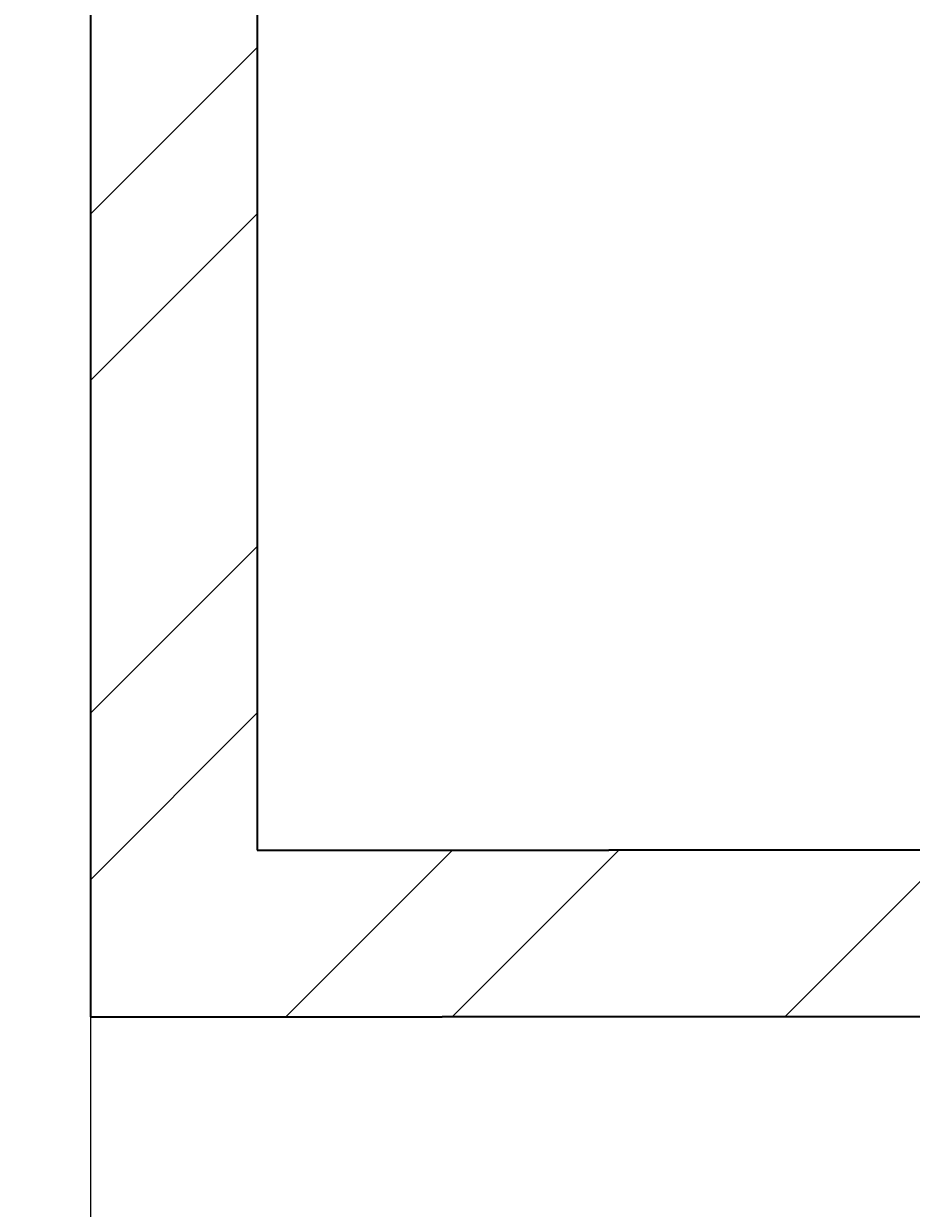
# Model space of a CAD drawing. Units: inches. Extents: x 1885 to 2748, y 783 to 2421.
# Tile 4 of 117: x 1969 to 1993, y 1082 to 1114. Entities that reach past the tile are written whole.
import ezdxf

# ---------------------------------------------------------------- set-up
doc = ezdxf.new("R2010")
doc.units = ezdxf.units.IN
for name, color, linetype, lineweight in [('A-ANNO-DIMS', 2, 'Continuous', 18), ('A-FLOR-BALC', 7, 'Continuous', 25), ('A-WALL', 7, 'Continuous', 35)]:
    doc.layers.add(name, color=color, linetype=linetype, lineweight=lineweight)
doc.layers.add('A-WALL-PATT', color=85, linetype='Continuous', lineweight=13, true_color=0x58ba48)
doc.styles.get("Standard").update_dxf_attribs({"font": 'arial.ttf'})
doc.dimstyles.get("Standard").update_dxf_attribs({"dimtxt": 0.18, "dimasz": 0.18, "dimexe": 0.18, "dimexo": 0.0625, "dimgap": 0.09, "dimtad": 0, "dimtih": 1, "dimtoh": 1, "dimdec": 4, "dimzin": 0, "dimdsep": 46, "dimtxsty": 'Standard', "dimcen": 0.09, "dimadec": 0, "dimazin": 0, "dimtfac": 1, "dimtdec": 4, "dimtofl": 0, "dimtmove": 0, "dimatfit": 3, "dimfxl": 1, "dimtolj": 1, "dimtzin": 0, "dimarcsym": 0})

# ---------------------------------------------------------------- blocks, each defined once
blk = doc.blocks.new('*D45')
at = {"layer": 'A-ANNO-DIMS', "color": 0, "lineweight": -2, "transparency": 16777216}
for p, q in [((1980.711, 1524.006), (1902.844, 1524.006)), ((1903.024, 1523.826), (1903.024, 1290.937)), ((1903.024, 1057.686), (1903.024, 1290.574)), ((1971.211, 1057.506), (1902.844, 1057.506))]:
    blk.add_line(p, q, dxfattribs=at)
at = {"layer": 'A-ANNO-DIMS', "color": 0, "transparency": 16777216}
for points in [[(1902.994, 1523.826), (1903.054, 1523.826), (1903.024, 1524.006)], [(1902.994, 1057.686), (1903.054, 1057.686), (1903.024, 1057.506)]]:
    blk.add_solid(points, dxfattribs=at)
at = {"layer": 'Defpoints', "color": 0, "transparency": 16777216}
for p in [(1903.024, 1524.006), (1980.774, 1524.006), (1971.274, 1057.506)]:
    blk.add_point(p, dxfattribs=at)
at = {"layer": 'A-ANNO-DIMS', "color": 0, "transparency": 16777216, "insert": (1903.024, 1290.756), "char_height": 0.18, "attachment_point": 5}
blk.add_mtext('\\A1;466.5', dxfattribs=at)

msp = doc.modelspace()

# ---------------------------------------------------------------- hatches: boundary and pattern name
at = {"layer": 'A-WALL-PATT'}
h = msp.add_hatch(dxfattribs=at)
h.set_pattern_fill('ANSI32', color=256)
h.paths.add_polyline_path([(2007.772, 2318.006), (1980.774, 2318.006), (1980.774, 2281.215), (1985.274, 2281.215), (1985.274, 2313.506), (2007.772, 2313.506), (2007.772, 2315.756)])
h.paths.add_polyline_path([(2094.324, 2318.006), (2067.772, 2318.006), (2067.772, 2313.506), (2094.324, 2313.506), (2094.324, 2315.756)])
h.paths.add_polyline_path([(2131.367, 2315.756), (2131.367, 2318.006), (2131.189, 2318.006), (2112.609, 2318.006), (2112.609, 2313.506), (2117.274, 2313.506), (2117.274, 2255.201), (2121.774, 2255.201), (2121.774, 2313.506), (2131.367, 2313.506)])
h.paths.add_polyline_path([(2190.512, 2318.006), (2155.367, 2318.006), (2155.367, 2313.506), (2169.774, 2313.506), (2169.774, 2229.506), (2121.774, 2229.506), (2121.774, 2233.451), (2119.524, 2233.451), (2117.274, 2233.451), (2117.274, 2201.101), (2121.774, 2201.101), (2121.774, 2225.006), (2169.774, 2225.006), (2169.774, 2165.006), (2306.274, 2165.006), (2306.274, 2066.006), (2310.774, 2066.006), (2344.274, 2066.006), (2486.274, 2066.006), (2486.274, 1886.006), (2483.02, 1886.006), (2483.02, 1881.506), (2486.274, 1881.506), (2486.274, 1880.678), (2490.774, 1880.678), (2490.774, 2070.506), (2344.274, 2070.506), (2310.774, 2070.506), (2310.774, 2165.006), (2310.774, 2173.636), (2308.524, 2173.636), (2306.274, 2173.636), (2306.274, 2169.506), (2174.274, 2169.506), (2174.274, 2313.506), (2190.512, 2313.506), (2190.512, 2315.756)])
h.paths.add_polyline_path([(1985.274, 2221.215), (1980.774, 2221.215), (1980.774, 2165.006), (1992.774, 2165.006), (1992.774, 2141.927), (1997.274, 2141.927), (1997.274, 2165.006), (2117.274, 2165.006), (2117.274, 2163.126), (2121.774, 2163.126), (2121.774, 2172.734), (2119.524, 2172.734), (2117.274, 2172.734), (2117.274, 2169.506), (1985.274, 2169.506)])
h.paths.add_polyline_path([(1997.274, 2105.927), (1992.774, 2105.927), (1992.774, 2070.506), (2016.774, 2070.506), (2016.774, 2059.123), (2019.024, 2059.123), (2021.274, 2059.123), (2021.274, 2070.506), (2117.274, 2070.506), (2117.274, 2022.506), (2114.423, 2022.506), (2114.423, 2018.006), (2123.627, 2018.006), (2123.627, 2020.256), (2123.627, 2022.506), (2121.774, 2022.506), (2121.774, 2142.587), (2119.524, 2142.587), (2117.274, 2142.587), (2117.274, 2075.006), (1997.274, 2075.006)])
h.paths.add_polyline_path([(2092.029, 2020.256), (2092.029, 2022.506), (2021.274, 2022.506), (2021.274, 2035.123), (2016.774, 2035.123), (2016.774, 2018.006), (2016.774, 1978.784), (2021.274, 1978.784), (2021.274, 2018.006), (2092.029, 2018.006)])
h.paths.add_polyline_path([(2260.938, 2022.506), (2153.105, 2022.506), (2153.105, 2020.256), (2153.105, 2018.006), (2155.274, 2018.006), (2155.274, 1886.006), (2107.629, 1886.006), (2107.629, 1881.506), (2182.911, 1881.506), (2182.911, 1883.756), (2182.911, 1886.006), (2159.774, 1886.006), (2159.774, 2018.006), (2260.938, 2018.006), (2260.938, 2020.256)])
h.paths.add_polyline_path([(2047.629, 1883.756), (2047.629, 1886.006), (2021.274, 1886.006), (2021.274, 1918.784), (2019.024, 1918.784), (2016.774, 1918.784), (2016.774, 1881.506), (2047.629, 1881.506)])
h.paths.add_polyline_path([(2306.361, 1883.756), (2306.361, 1886.006), (2296.274, 1886.006), (2296.274, 1982.006), (2316.535, 1982.006), (2316.535, 1984.256), (2316.535, 1986.506), (2296.274, 1986.506), (2296.274, 2022.506), (2289.276, 2022.506), (2289.276, 2018.006), (2291.774, 2018.006), (2291.774, 1886.006), (2242.911, 1886.006), (2242.911, 1881.506), (2306.361, 1881.506)], flags=17)
h.paths.add_polyline_path([(1985.274, 1843.006), (2021.6, 1843.006), (2021.534, 1845.441), (2021.477, 1847.506), (1980.774, 1847.506), (1980.774, 1809.446), (1985.274, 1809.446)])
h.paths.add_polyline_path([(2131.482, 1845.256), (2131.482, 1847.506), (2081.534, 1847.506), (2081.534, 1843.006), (2117.274, 1843.006), (2117.274, 1784.147), (2119.524, 1784.147), (2121.774, 1784.147), (2121.774, 1843.006), (2131.482, 1843.006)])
h.paths.add_polyline_path([(2203.886, 1847.506), (2155.482, 1847.506), (2155.482, 1843.006), (2169.774, 1843.006), (2169.774, 1759.006), (2121.774, 1759.006), (2121.774, 1761.457), (2117.274, 1761.457), (2117.274, 1730.429), (2121.774, 1730.429), (2121.774, 1754.506), (2177.421, 1754.506), (2177.421, 1756.756), (2177.421, 1759.006), (2174.274, 1759.006), (2174.274, 1843.006), (2203.886, 1843.006)])
h.paths.add_polyline_path([(2335.554, 1845.256), (2335.554, 1847.506), (2239.886, 1847.506), (2239.886, 1843.006), (2306.274, 1843.006), (2306.274, 1759.006), (2199.486, 1759.006), (2199.486, 1754.506), (2310.774, 1754.506), (2310.774, 1843.006), (2335.554, 1843.006)])
h.paths.add_polyline_path([(2348.774, 2022.506), (2344.274, 2022.506), (2344.274, 1986.506), (2341.681, 1986.506), (2341.681, 1982.006), (2344.274, 1982.006), (2344.274, 1886.006), (2330.361, 1886.006), (2330.361, 1881.506), (2361.627, 1881.506), (2361.627, 1883.756), (2361.627, 1886.006), (2348.774, 1886.006)], flags=17)
h.paths.add_polyline_path([(2283.251, 2315.756), (2283.251, 2318.006), (2238.512, 2318.006), (2238.512, 2313.506), (2283.251, 2313.506)], flags=17)
h.paths.add_polyline_path([(2363.274, 2348.006), (2388.677, 2348.006), (2388.677, 2350.256), (2388.677, 2352.506), (2358.774, 2352.506), (2358.774, 2348.006), (2358.774, 2318.006), (2344.481, 2318.006), (2344.481, 2313.506), (2358.774, 2313.506), (2358.774, 2229.506), (2310.774, 2229.506), (2310.774, 2231.952), (2306.274, 2231.952), (2306.274, 2205.611), (2310.774, 2205.611), (2310.774, 2225.006), (2358.774, 2225.006), (2358.774, 2211.506), (2452.329, 2211.506), (2452.329, 2213.756), (2452.329, 2216.006), (2363.274, 2216.006), (2363.274, 2318.006)])
h.paths.add_polyline_path([(2310.774, 2313.506), (2320.481, 2313.506), (2320.481, 2315.756), (2320.481, 2318.006), (2302.728, 2318.006), (2302.728, 2313.506), (2306.274, 2313.506), (2306.274, 2251.076), (2310.774, 2251.076)], flags=17)
h.paths.add_polyline_path([(2490.774, 2352.506), (2486.274, 2352.506), (2448.677, 2352.506), (2448.677, 2348.006), (2486.274, 2348.006), (2486.274, 2318.006), (2486.274, 2216.006), (2481.78, 2216.006), (2481.78, 2211.506), (2486.274, 2211.506), (2486.274, 2165.006), (2493.289, 2165.006), (2493.289, 2167.256), (2493.289, 2169.506), (2490.774, 2169.506), (2490.774, 2313.506), (2494.429, 2313.506), (2494.429, 2318.006), (2490.774, 2318.006)])
h.paths.add_polyline_path([(2534.653, 2318.006), (2515.691, 2318.006), (2515.691, 2313.506), (2534.653, 2313.506), (2534.653, 2315.756)])
h.paths.add_polyline_path([(2618.274, 2318.006), (2594.653, 2318.006), (2594.653, 2313.506), (2613.774, 2313.506), (2613.774, 2281.706), (2618.274, 2281.706)])
h.paths.add_polyline_path([(2618.274, 2221.706), (2613.774, 2221.706), (2613.774, 2169.506), (2554.019, 2169.506), (2554.019, 2165.006), (2613.774, 2165.006), (2613.774, 2152.878), (2618.274, 2152.878)])
h.paths.add_polyline_path([(2618.274, 2128.878), (2616.024, 2128.878), (2613.774, 2128.878), (2613.774, 2117.006), (2529.774, 2117.006), (2529.774, 2165.006), (2532.848, 2165.006), (2532.848, 2169.506), (2522.867, 2169.506), (2522.867, 2165.006), (2525.274, 2165.006), (2525.274, 2117.006), (2525.274, 2112.506), (2525.274, 2108.576), (2529.774, 2108.576), (2529.774, 2112.506), (2613.774, 2112.506), (2613.774, 2080.19), (2618.274, 2080.19)])
h.paths.add_polyline_path([(2618.274, 2044.19), (2616.024, 2044.19), (2613.774, 2044.19), (2613.774, 2015.506), (2529.774, 2015.506), (2529.774, 2088.582), (2527.524, 2088.582), (2525.274, 2088.582), (2525.274, 2011.006), (2613.774, 2011.006), (2613.774, 1956.755), (2618.274, 1956.755)])
h.paths.add_polyline_path([(2618.274, 1881.506), (2618.274, 1896.755), (2613.774, 1896.755), (2613.774, 1881.506), (2613.774, 1847.506), (2592.715, 1847.506), (2592.715, 1843.006), (2613.774, 1843.006), (2613.774, 1765.006), (2613.774, 1760.506), (2609.621, 1760.506), (2609.621, 1756.006), (2613.774, 1756.006), (2613.774, 1660.006), (2608.544, 1660.006), (2608.544, 1655.506), (2613.774, 1655.506), (2613.774, 1508.158), (2618.274, 1508.158)])
h.paths.add_polyline_path([(2565.774, 1843.006), (2568.997, 1843.006), (2568.997, 1847.506), (2490.774, 1847.506), (2490.774, 1849.7), (2488.524, 1849.7), (2486.274, 1849.7), (2486.274, 1847.506), (2477.274, 1847.506), (2477.274, 1838.506), (2477.274, 1821.493), (2486.274, 1821.493), (2486.274, 1838.506), (2561.274, 1838.506), (2561.274, 1765.006), (2486.274, 1765.006), (2486.274, 1786.157), (2477.274, 1786.157), (2477.274, 1765.006), (2477.274, 1756.006), (2486.274, 1756.006), (2565.774, 1756.006), (2585.621, 1756.006), (2585.621, 1758.256), (2585.621, 1760.506), (2565.774, 1760.506), (2565.774, 1765.006)])
h.paths.add_polyline_path([(2486.274, 1651.006), (2561.274, 1651.006), (2561.274, 1567.006), (2486.274, 1567.006), (2486.274, 1591.321), (2477.274, 1591.321), (2477.274, 1567.006), (2477.274, 1558.006), (2477.274, 1555.439), (2481.774, 1555.439), (2481.774, 1558.006), (2568.653, 1558.006), (2568.653, 1560.256), (2568.653, 1562.506), (2565.774, 1562.506), (2565.774, 1655.506), (2584.544, 1655.506), (2584.544, 1657.756), (2584.544, 1660.006), (2565.774, 1660.006), (2486.274, 1660.006), (2477.274, 1660.006), (2477.274, 1651.006), (2477.274, 1632.989), (2486.274, 1632.989)])
h.paths.add_polyline_path([(2449.967, 1883.756), (2449.967, 1886.006), (2421.627, 1886.006), (2421.627, 1881.506), (2449.967, 1881.506)], flags=17)
h.paths.add_polyline_path([(2447.274, 1847.506), (2395.554, 1847.506), (2395.554, 1843.006), (2442.774, 1843.006), (2442.774, 1809.27), (2447.274, 1809.27)])
h.paths.add_polyline_path([(1985.274, 1749.446), (1980.774, 1749.446), (1980.774, 1694.504), (1985.274, 1694.504), (1985.274, 1694.506), (1986.897, 1694.506), (1986.897, 1697.78), (1986.897, 1699.006), (1985.274, 1699.006)])
h.paths.add_polyline_path([(2152.774, 1699.006), (2121.774, 1699.006), (2121.774, 1703.668), (2119.524, 1703.668), (2117.274, 1703.668), (2117.274, 1699.006), (2009.219, 1699.006), (2009.219, 1694.506), (2148.274, 1694.506), (2148.274, 1692.631), (2152.774, 1692.631)])
h.paths.add_polyline_path([(2016.274, 1694.506), (2011.774, 1694.506), (2011.774, 1558.006), (2040.806, 1558.006), (2040.806, 1560.256), (2040.806, 1562.506), (2016.274, 1562.506)])
h.paths.add_polyline_path([(2152.774, 1663.017), (2150.524, 1663.017), (2148.274, 1663.017), (2148.274, 1562.506), (2100.806, 1562.506), (2100.806, 1558.006), (2165.119, 1558.006), (2165.119, 1560.256), (2165.119, 1562.506), (2152.774, 1562.506), (2152.774, 1610.506), (2224.774, 1610.506), (2224.774, 1607.99), (2229.274, 1607.99), (2229.274, 1615.006), (2152.774, 1615.006)])
h.paths.add_polyline_path([(2238.613, 1560.256), (2238.613, 1562.506), (2229.274, 1562.506), (2229.274, 1588.756), (2227.024, 1588.763), (2224.774, 1588.771), (2224.774, 1562.506), (2189.119, 1562.506), (2189.119, 1558.006), (2238.613, 1558.006)])
h.paths.add_polyline_path([(2336.024, 1560.256), (2336.024, 1562.506), (2310.774, 1562.506), (2310.774, 1656.347), (2308.524, 1656.347), (2306.274, 1656.347), (2306.274, 1562.506), (2286.613, 1562.506), (2286.613, 1558.006), (2336.024, 1558.006)])
h.paths.add_polyline_path([(2447.274, 1690.968), (2445.024, 1690.968), (2442.774, 1690.968), (2442.774, 1687.006), (2306.274, 1687.006), (2306.274, 1680.75), (2310.774, 1680.75), (2310.774, 1682.506), (2442.774, 1682.506), (2442.774, 1562.506), (2396.024, 1562.506), (2396.024, 1558.006), (2447.274, 1558.006)])
h.paths.add_polyline_path([(2447.274, 1749.27), (2445.024, 1749.27), (2442.774, 1749.27), (2442.774, 1717.232), (2447.274, 1717.232)])
h.paths.add_polyline_path([(2044.674, 1521.756), (2044.674, 1524.006), (2007.274, 1524.006), (2007.274, 1503.49), (2009.524, 1503.49), (2011.774, 1503.49), (2011.774, 1519.506), (2044.674, 1519.506)])
h.paths.add_polyline_path([(2177.969, 1521.756), (2177.969, 1524.006), (2104.674, 1524.006), (2104.674, 1519.506), (2145.774, 1519.506), (2145.774, 1387.506), (2143.37, 1387.506), (2143.37, 1383.006), (2251.585, 1383.006), (2251.585, 1385.256), (2251.585, 1387.506), (2150.274, 1387.506), (2150.274, 1519.506), (2177.969, 1519.506)])
h.paths.add_polyline_path([(2298.704, 1524.006), (2237.969, 1524.006), (2237.969, 1519.506), (2282.274, 1519.506), (2282.274, 1387.506), (2279.683, 1387.506), (2279.683, 1383.006), (2286.774, 1383.006), (2286.774, 1419.006), (2312.451, 1419.006), (2312.451, 1421.256), (2312.451, 1423.506), (2286.774, 1423.506), (2286.774, 1519.506), (2298.704, 1519.506), (2298.704, 1521.722)], flags=17)
h.paths.add_polyline_path([(2361.897, 1521.756), (2361.897, 1524.006), (2322.704, 1524.006), (2322.704, 1519.506), (2334.774, 1519.506), (2334.774, 1423.506), (2331.93, 1423.506), (2331.93, 1419.006), (2334.774, 1419.006), (2334.774, 1387.506), (2334.774, 1383.228), (2339.274, 1383.228), (2339.274, 1387.506), (2339.274, 1519.506), (2361.897, 1519.506)], flags=17)
h.paths.add_polyline_path([(2447.274, 1521.756), (2447.274, 1524.006), (2421.897, 1524.006), (2421.897, 1519.506), (2447.274, 1519.506)], flags=17)
h.paths.add_polyline_path([(2481.774, 1529.6), (2479.524, 1529.6), (2477.274, 1529.6), (2477.274, 1524.006), (2474.489, 1524.006), (2474.489, 1519.506), (2477.274, 1519.506), (2477.274, 1334.506), (2296.774, 1334.506), (2296.774, 1240.506), (2160.274, 1240.506), (2160.274, 1180.506), (2112.274, 1180.506), (2112.274, 1207.692), (2110.024, 1207.692), (2107.774, 1207.692), (2107.774, 1171.609), (2112.274, 1171.609), (2112.274, 1176.006), (2160.274, 1176.006), (2160.274, 1092.006), (2144.221, 1092.006), (2144.221, 1087.506), (2189.497, 1087.506), (2189.497, 1089.756), (2189.497, 1092.006), (2164.774, 1092.006), (2164.774, 1236.006), (2296.774, 1236.006), (2296.774, 1231.912), (2301.274, 1231.912), (2301.274, 1330.006), (2481.774, 1330.006), (2481.774, 1387.506)])
h.paths.add_polyline_path([(2618.274, 1448.158), (2613.774, 1448.158), (2613.774, 1382.506), (2529.774, 1382.506), (2525.274, 1382.506), (2525.274, 1307.062), (2529.774, 1307.062), (2529.774, 1378.006), (2613.774, 1378.006), (2613.774, 1354.988), (2618.274, 1354.988)])
h.paths.add_polyline_path([(2618.274, 1318.988), (2613.774, 1318.988), (2613.774, 1281.006), (2529.774, 1281.006), (2529.774, 1283.786), (2527.524, 1283.786), (2525.274, 1283.786), (2525.274, 1228.506), (2516.794, 1228.506), (2516.794, 1224.006), (2533.484, 1224.006), (2533.484, 1226.256), (2533.484, 1228.506), (2529.774, 1228.506), (2529.774, 1276.506), (2613.774, 1276.506), (2613.774, 1266.02), (2618.274, 1266.02)])
h.paths.add_polyline_path([(2618.274, 1134.964), (2613.774, 1134.964), (2613.774, 1092.006), (2594.545, 1092.006), (2594.545, 1087.506), (2618.274, 1087.506)])
h.paths.add_polyline_path([(2534.545, 1092.006), (2509.765, 1092.006), (2509.765, 1087.506), (2534.545, 1087.506), (2534.545, 1089.756)])
h.paths.add_polyline_path([(2481.274, 1224.006), (2484.117, 1224.006), (2484.117, 1226.256), (2484.117, 1228.506), (2476.774, 1228.506), (2476.774, 1198.506), (2471.61, 1198.506), (2471.61, 1194.006), (2476.774, 1194.006), (2476.774, 1062.006), (2436.894, 1062.006), (2436.894, 1057.506), (2476.774, 1057.506), (2481.274, 1057.506), (2481.274, 1062.006), (2481.274, 1087.506), (2485.354, 1087.506), (2485.354, 1089.756), (2485.354, 1092.006), (2481.274, 1092.006), (2481.274, 1117.506)])
h.paths.add_polyline_path([(2439.898, 1198.506), (2349.274, 1198.506), (2349.274, 1194.006), (2349.274, 1180.506), (2301.274, 1180.506), (2301.274, 1201.896), (2299.024, 1201.896), (2296.774, 1201.896), (2296.774, 1172.335), (2299.024, 1172.335), (2301.274, 1172.335), (2301.274, 1176.006), (2349.274, 1176.006), (2349.274, 1092.006), (2334.452, 1092.006), (2334.452, 1087.506), (2349.274, 1087.506), (2349.274, 1057.506), (2353.774, 1057.506), (2376.894, 1057.506), (2376.894, 1059.756), (2376.894, 1062.006), (2353.774, 1062.006), (2353.774, 1087.506), (2353.774, 1180.506), (2353.774, 1194.006), (2439.898, 1194.006), (2439.898, 1196.256)])
h.paths.add_polyline_path([(2270.596, 1089.756), (2270.596, 1092.006), (2249.497, 1092.006), (2249.497, 1087.506), (2270.596, 1087.506)], flags=17)
h.paths.add_polyline_path([(2310.452, 1092.006), (2301.274, 1092.006), (2301.274, 1153.292), (2296.774, 1153.292), (2296.774, 1092.006), (2293.786, 1092.006), (2293.786, 1087.506), (2310.452, 1087.506), (2310.452, 1089.756)], flags=17)
h.paths.add_polyline_path([(2112.274, 1150.328), (2110.024, 1150.328), (2107.774, 1150.328), (2107.774, 1092.006), (2104.465, 1092.006), (2104.465, 1087.506), (2120.221, 1087.506), (2120.221, 1089.756), (2120.221, 1092.006), (2112.274, 1092.006)])
h.paths.add_polyline_path([(2082.172, 1092.006), (2058.144, 1092.006), (2058.144, 1087.506), (2082.172, 1087.506), (2082.172, 1089.756)])
h.paths.add_polyline_path([(1975.774, 1145.638), (1971.274, 1145.638), (1971.274, 1087.506), (1980.774, 1087.506), (1998.144, 1087.506), (1998.144, 1089.756), (1998.144, 1092.006), (1985.274, 1092.006), (1975.774, 1092.006)])
h.paths.add_polyline_path([(2112.274, 1244.385), (2110.024, 1244.385), (2107.774, 1244.385), (2107.774, 1240.506), (1992.274, 1240.506), (1992.274, 1271.008), (1987.774, 1271.008), (1987.774, 1240.506), (1980.774, 1240.506), (1975.774, 1240.506), (1971.274, 1240.506), (1971.274, 1205.638), (1975.774, 1205.638), (1975.774, 1236.006), (2107.774, 1236.006), (2107.774, 1233.444), (2112.274, 1233.444), (2112.274, 1236.006)])
h.paths.add_polyline_path([(2112.274, 1383.006), (2114.783, 1383.006), (2114.783, 1385.256), (2114.783, 1387.506), (2102.476, 1387.506), (2102.476, 1383.006), (2107.774, 1383.006), (2107.774, 1335.006), (2011.774, 1335.006), (2011.774, 1349.939), (2007.274, 1349.939), (2007.274, 1335.006), (1987.774, 1335.006), (1987.774, 1330.506), (1987.774, 1307.008), (1992.274, 1307.008), (1992.274, 1330.506), (2007.274, 1330.506), (2107.774, 1330.506), (2107.774, 1264.711), (2112.274, 1264.711)])
h.paths.add_polyline_path([(2077.857, 1387.506), (2011.774, 1387.506), (2011.774, 1390.036), (2009.524, 1390.036), (2007.274, 1390.036), (2007.274, 1373.939), (2011.774, 1373.939), (2011.774, 1383.006), (2077.857, 1383.006)])
h.paths.add_polyline_path([(2011.774, 1443.49), (2007.274, 1443.49), (2007.274, 1410.248), (2011.774, 1410.248)])

# ---------------------------------------------------------------- linework, layer by layer
at = {"layer": 'A-FLOR-BALC'}
msp.add_line((1971.274, 1087.506), (1971.274, 1057.506), dxfattribs=at)
at = {"layer": 'A-WALL'}
for p, q in [((1971.274, 1145.638), (1971.274, 1087.506)), ((1975.774, 1145.638), (1975.774, 1092.006)), ((1975.774, 1092.006), (1985.274, 1092.006)), ((1998.144, 1092.006), (1985.274, 1092.006)), ((1971.274, 1087.506), (1980.774, 1087.506)), ((1998.144, 1087.506), (1980.774, 1087.506))]:
    msp.add_line(p, q, dxfattribs=at)

# ---------------------------------------------------------------- dimensions: what is measured, and where the dimension line sits
at = {"layer": 'A-ANNO-DIMS'}
dim = msp.add_linear_dim(base=(1903.024, 1524.006), p1=(1971.274, 1057.506), p2=(1980.774, 1524.006), angle=90, dimstyle='Standard', override={"dimdec": 1, "dimlfac": 1, "dimrnd": 0, "dimzin": 0, "dimdsep": 46, "dimlunit": 2}, dxfattribs=at)
dim.commit()
dim.dimension.update_dxf_attribs({"geometry": '*D45', "text_midpoint": (1903.024, 1290.756)})

doc.saveas('drawing.dxf')
